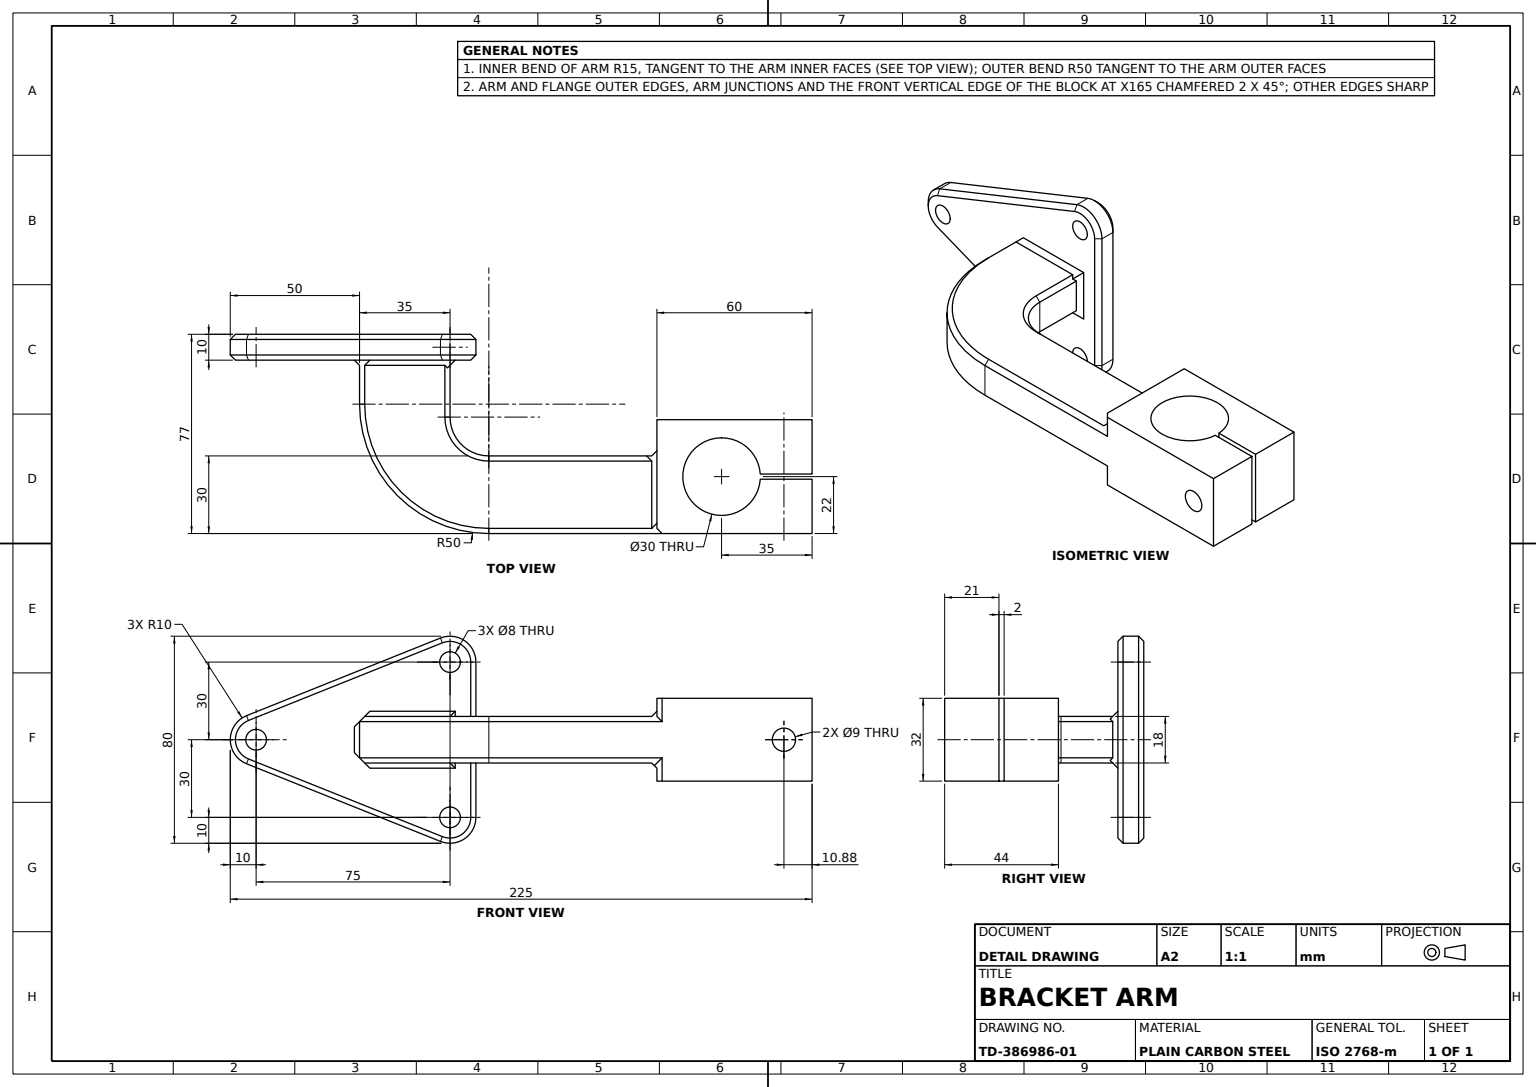
from build123d import *

# Parameters (mm, degrees)
CLAMP_BLOCK_SKETCH_W       = 60
CLAMP_BLOCK_SKETCH_H       = 32
CLAMP_BLOCK_DEPTH          = 44
SPLIT_BORE_CUT_DEPTH       = 44
CLAMP_BOLT_HOLE_SKETCH_R   = 4.5
CLAMP_BOLT_HOLE_DEPTH      = 60
ARM_SKETCH_W               = 30
ARM_SKETCH_H               = 18
ARM_DEPTH                  = 65
ARM_BEND_DEPTH             = 18
MOUNTING_FLANGE_DEPTH      = 10
FLANGE_HOLES_SKETCH_R      = 4
FLANGE_HOLES_3X_8_DEPTH    = 10
ARM_BEND_CHAMFER_SIZE      = 2
CLAMP_BLOCK_CHAMFER_A_SIZE = 2
ARM_CLAMP_CHAMFER_A_SIZE   = 2
ARM_EDGE_CHAMFER_SIZE      = 2
ARM_CLAMP_CHAMFER_B_SIZE   = 2
CLAMP_BLOCK_CHAMFER_B_SIZE = 2
ARM_FLANGE_CHAMFER_A_SIZE  = 2
BEND_FLANGE_CHAMFER_A_SIZE = 2
ARM_FLANGE_CHAMFER_B_SIZE  = 2
BEND_FLANGE_CHAMFER_B_SIZE = 2
FLANGE_EDGE_CHAMFER_SIZE   = 2
BEND_EDGE_CHAMFER_A_SIZE   = 2
BEND_EDGE_CHAMFER_B_SIZE   = 2
ARM_CLAMP_CHAMFER_C_SIZE   = 2


with BuildPart() as part:
    # Clamp Block Sketch → Clamp Block (new body)
    with BuildSketch(Plane.XY):
        with Locations((30, -16)):
            Rectangle(CLAMP_BLOCK_SKETCH_W, CLAMP_BLOCK_SKETCH_H)
    extrude(amount=-CLAMP_BLOCK_DEPTH)

    # Split Bore Sketch → Split Bore Cut (cut)
    with BuildSketch(Plane.XZ.offset(32)):
        with BuildLine():
            Line((60, -21), (60, -23))
            Line((60, -23), (39.966629547, -23))
            ThreePointArc((39.966629547, -23), (10, -22), (39.966629547, -21))
            Line((39.966629547, -21), (60, -21))
        make_face()
    extrude(amount=-SPLIT_BORE_CUT_DEPTH, mode=Mode.SUBTRACT)

    # Clamp Bolt Hole Sketch → Clamp Bolt Hole (cut)
    with BuildSketch(Plane.XY):
        with Locations(Location((49.119785918, -16, 0), (0, 0, 180))):
            Circle(CLAMP_BOLT_HOLE_SKETCH_R)
    extrude(amount=-CLAMP_BOLT_HOLE_DEPTH, mode=Mode.SUBTRACT)

    # Arm Sketch → Arm (add)
    with BuildSketch(Plane.ZY):
        with Locations((-15, -16)):
            Rectangle(ARM_SKETCH_W, ARM_SKETCH_H)
    extrude(amount=ARM_DEPTH)

    # Arm Bend Sketch → Arm Bend (add)
    with BuildSketch(Plane.XZ.offset(25)):
        with BuildLine():
            Line((-115, -67), (-80, -67))
            Line((-80, -67), (-80, -45))
            ThreePointArc((-80, -45), (-75.606601718, -34.393398282), (-65, -30))
            Line((-65, -30), (-65, 0))
            ThreePointArc((-65, 0), (-100.355339059, -14.644660941), (-115, -50))
            Line((-115, -50), (-115, -67))
        make_face()
    extrude(amount=-ARM_BEND_DEPTH)

    # Mounting Flange Sketch → Mounting Flange (add)
    with BuildSketch(Plane(origin=(0, 0, -67), x_dir=(-1, 0, 0), z_dir=(0, 0, -1))):
        with BuildLine():
            Line((83.713906764, 23.284766909), (158.713906764, -6.715233091))
            ThreePointArc((158.713906764, -6.715233091), (165, -16), (158.713906764, -25.284766909))
            Line((158.713906764, -25.284766909), (83.713906764, -55.284766909))
            ThreePointArc((83.713906764, -55.284766909), (74.393711907, -54.280672305), (70, -46))
            Line((70, -46), (70, 14))
            ThreePointArc((70, 14), (74.393711907, 22.280672305), (83.713906764, 23.284766909))
        make_face()
    extrude(amount=MOUNTING_FLANGE_DEPTH)

    # Flange Holes Sketch → Flange Holes 3xØ8 (cut)
    with BuildSketch(Plane(origin=(0, 0, -77), x_dir=(-1, 0, 0), z_dir=(0, 0, -1))):
        with Locations((80, 14)):
            Circle(FLANGE_HOLES_SKETCH_R)
        with Locations((155, -16)):
            Circle(FLANGE_HOLES_SKETCH_R)
        with Locations((80, -46)):
            Circle(FLANGE_HOLES_SKETCH_R)
    extrude(amount=-FLANGE_HOLES_3X_8_DEPTH, mode=Mode.SUBTRACT)

    # Arm-Bend Chamfer
    arm_bend_chamfer_edges = [part.edges().sort_by_distance(p)[0] for p in [
        (-32.5, -25, 0),
        (-100.355339059, -25, -14.644660941),
        (-115, -25, -58.5),
    ]]
    chamfer(arm_bend_chamfer_edges, length=ARM_BEND_CHAMFER_SIZE)

    # Clamp Block Chamfer A
    clamp_block_chamfer_a_edges = [part.edges().sort_by_distance(p)[0] for p in [
        (0, -27.5, 0),
    ]]
    chamfer(clamp_block_chamfer_a_edges, length=CLAMP_BLOCK_CHAMFER_A_SIZE)

    # Arm-Clamp Chamfer A
    arm_clamp_chamfer_a_edges = [part.edges().sort_by_distance(p)[0] for p in [
        (0, -25, -16),
    ]]
    chamfer(arm_clamp_chamfer_a_edges, length=ARM_CLAMP_CHAMFER_A_SIZE)

    # Arm Edge Chamfer
    arm_edge_chamfer_edges = [part.edges().sort_by_distance(p)[0] for p in [
        (-32.5, -7, 0),
        (-115, -7, -58.5),
        (-100.355339059, -7, -14.644660941),
    ]]
    chamfer(arm_edge_chamfer_edges, length=ARM_EDGE_CHAMFER_SIZE)

    # Arm-Clamp Chamfer B
    arm_clamp_chamfer_b_edges = [part.edges().sort_by_distance(p)[0] for p in [
        (0, -7, -16),
    ]]
    chamfer(arm_clamp_chamfer_b_edges, length=ARM_CLAMP_CHAMFER_B_SIZE)

    # Clamp Block Chamfer B
    clamp_block_chamfer_b_edges = [part.edges().sort_by_distance(p)[0] for p in [
        (0, -4.5, 0),
    ]]
    chamfer(clamp_block_chamfer_b_edges, length=CLAMP_BLOCK_CHAMFER_B_SIZE)

    # Arm-Flange Chamfer A
    arm_flange_chamfer_a_edges = [part.edges().sort_by_distance(p)[0] for p in [
        (-96.5, -25, -67),
        (-74.393711907, 22.280672305, -67),
        (-70, -16, -67),
        (-74.393711907, -54.280672305, -67),
        (-121.213906764, -40.284766909, -67),
        (-165, -16, -67),
        (-121.213906764, 8.284766909, -67),
    ]]
    chamfer(arm_flange_chamfer_a_edges, length=ARM_FLANGE_CHAMFER_A_SIZE)

    # Bend-Flange Chamfer A
    bend_flange_chamfer_a_edges = [part.edges().sort_by_distance(p)[0] for p in [
        (-115, -16, -67),
    ]]
    chamfer(bend_flange_chamfer_a_edges, length=BEND_FLANGE_CHAMFER_A_SIZE)

    # Arm-Flange Chamfer B
    arm_flange_chamfer_b_edges = [part.edges().sort_by_distance(p)[0] for p in [
        (-96.5, -7, -67),
    ]]
    chamfer(arm_flange_chamfer_b_edges, length=ARM_FLANGE_CHAMFER_B_SIZE)

    # Bend-Flange Chamfer B
    bend_flange_chamfer_b_edges = [part.edges().sort_by_distance(p)[0] for p in [
        (-80, -16, -67),
    ]]
    chamfer(bend_flange_chamfer_b_edges, length=BEND_FLANGE_CHAMFER_B_SIZE)

    # Flange Edge Chamfer
    flange_edge_chamfer_edges = [part.edges().sort_by_distance(p)[0] for p in [
        (-74.393711907, 22.280672305, -77),
        (-70, -16, -77),
        (-74.393711907, -54.280672305, -77),
        (-121.213906764, -40.284766909, -77),
        (-165, -16, -77),
        (-121.213906764, 8.284766909, -77),
    ]]
    chamfer(flange_edge_chamfer_edges, length=FLANGE_EDGE_CHAMFER_SIZE)

    # Bend Edge Chamfer A
    bend_edge_chamfer_a_edges = [part.edges().sort_by_distance(p)[0] for p in [
        (-80, -25, -55),
        (-33.5, -25, -30),
        (-75.606601718, -25, -34.393398282),
    ]]
    chamfer(bend_edge_chamfer_a_edges, length=BEND_EDGE_CHAMFER_A_SIZE)

    # Bend Edge Chamfer B
    bend_edge_chamfer_b_edges = [part.edges().sort_by_distance(p)[0] for p in [
        (-80, -7, -55),
        (-33.5, -7, -30),
        (-75.606601718, -7, -34.393398282),
    ]]
    chamfer(bend_edge_chamfer_b_edges, length=BEND_EDGE_CHAMFER_B_SIZE)

    # Arm-Clamp Chamfer C
    arm_clamp_chamfer_c_edges = [part.edges().sort_by_distance(p)[0] for p in [
        (0, -16, -30),
    ]]
    chamfer(arm_clamp_chamfer_c_edges, length=ARM_CLAMP_CHAMFER_C_SIZE)


solid = part.part
